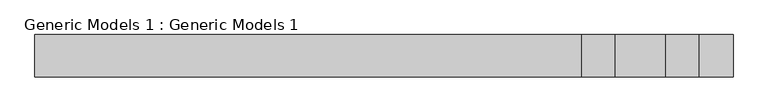
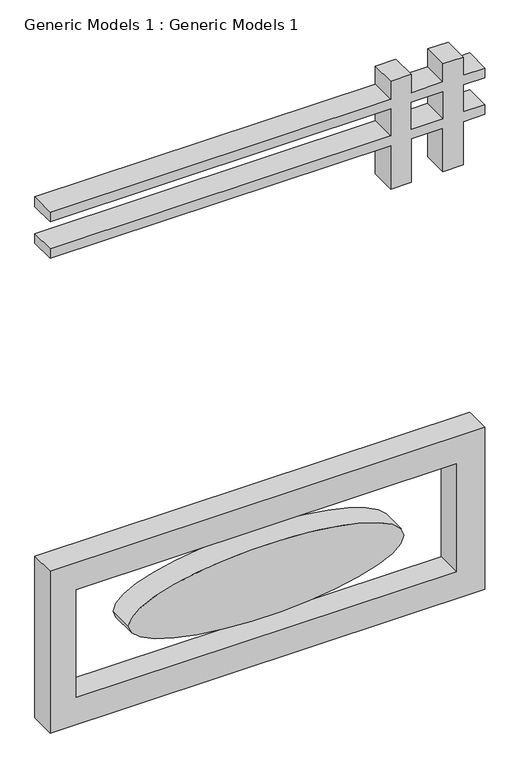
"""IFC4 building model written with IfcOpenShell, lengths in millimetres: proxy geometry, Generic Models 1 : Generic Models 1."""

from ifc_helpers import new_model, si_unit, point, frame, origin, place, context, project, spatial, polyline, ellipse_curve, trimmed, outline, extrude, source, transform, mapped, element, save
from ifc_brep_helpers import plane_surface, extruded_surface, advanced_brep


def generic_models_1_generic_models_1_d084bfd0(model_context):
    return source(origin(), model_context, "Body", "SolidModel", [
        extrude(outline(polyline([(2945.7806147, -9147.962181), (3048.0, -9147.962181), (3048.0, -9256.9307419), (2945.7806147, -9256.9307419), (2945.7806147, -9427.362181), (3048.0, -9427.362181), (3048.0, -9536.3307419), (2945.7806147, -9536.3307419), (2945.7806147, -11357.3277598), (2891.0724485, -11357.3277598), (2891.0724485, -9536.3307419), (2738.6724485, -9536.3307419), (2738.6724485, -11357.3277598), (2683.9642823, -11357.3277598), (2683.9642823, -9536.3307419), (2438.4, -9536.3307419), (2438.4, -9427.362181), (2683.9642823, -9427.362181), (2683.9642823, -9256.9307419), (2438.4, -9256.9307419), (2438.4, -9147.962181), (2683.9642823, -9147.962181), (2683.9642823, -9033.2277598), (2738.6724485, -9033.2277598), (2738.6724485, -9147.962181), (2891.0724485, -9147.962181), (2891.0724485, -9033.2277598), (2945.7806147, -9033.2277598), (2945.7806147, -9147.962181)]), holes=[polyline([(2738.6724485, -9427.362181), (2891.0724485, -9427.362181), (2891.0724485, -9256.9307419), (2738.6724485, -9256.9307419), (2738.6724485, -9427.362181)])]), frame((0.0, 2074.8342801, 0.0), z_axis=(0.0, 1.0, 0.0), x_axis=(0.0, 0.0, 1.0)), (0.0, 0.0, 1.0), 140.9087581),
        advanced_brep(
        [(-10938.2277598, 2074.8342801, 457.2), (-9465.0277598, 2074.8342801, 457.2), (-10938.2277598, 2215.7430382, 457.2), (-9465.0277598, 2215.7430382, 457.2)],
        [
            (0, 1, ellipse_curve(frame((-10201.6277598, 2074.8342801, 457.2), z_axis=(0.0, -1.0, 0.0), x_axis=(1.0, 0.0, 0.0)), 736.6, 203.2)),
            (1, 0, ellipse_curve(frame((-10201.6277598, 2074.8342801, 457.2), z_axis=(0.0, -1.0, 0.0), x_axis=(1.0, 0.0, 0.0)), 736.6, 203.2)),
            (2, 3, ellipse_curve(frame((-10201.6277598, 2215.7430382, 457.2), z_axis=(0.0, 1.0, 0.0), x_axis=(1.0, 0.0, 0.0)), 736.6, 203.2)),
            (3, 2, ellipse_curve(frame((-10201.6277598, 2215.7430382, 457.2), z_axis=(0.0, 1.0, 0.0), x_axis=(1.0, 0.0, 0.0)), 736.6, 203.2)),
            (0, 2),
            (3, 1),
        ],
        [
            plane_surface(frame((-9465.0277598, 2074.8342801, 457.2), z_axis=(0.0, -1.0, 0.0), x_axis=(0.0, 0.0, 1.0))),
            plane_surface(frame((-9465.0277598, 2215.7430382, 457.2), z_axis=(0.0, 1.0, 0.0), x_axis=(0.0, 0.0, -1.0))),
            extruded_surface(trimmed(ellipse_curve(frame((-10201.6277598, 2356.6517963, 457.2), z_axis=(0.0, -1.0, 0.0), x_axis=(1.0, 0.0, 0.0)), 736.6, 203.2), [point((-10938.2277598, 2356.6517963, 457.2))], [point((-9465.0277598, 2356.6517963, 457.2))], True, "CARTESIAN"), (0.0, -140.90875810000034, 0.0), 140.90875810000034),
            extruded_surface(trimmed(ellipse_curve(frame((-10201.6277598, 2356.6517963, 457.2), z_axis=(0.0, -1.0, 0.0), x_axis=(1.0, 0.0, 0.0)), 736.6, 203.2), [point((-9465.0277598, 2356.6517963, 457.2))], [point((-10938.2277598, 2356.6517963, 457.2))], True, "CARTESIAN"), (0.0, -140.90875810000034, 0.0), 140.90875810000034),
        ],
        [
            (0, [[1, 2]]),
            (1, [[3, 4]]),
            (2, [[-1, 5, -4, 6]]),
            (3, [[-2, -6, -3, -5]]),
        ],
    ),
        extrude(outline(polyline([(914.4, -11357.3277598), (0.0, -11357.3277598), (0.0, -9033.2277598), (914.4, -9033.2277598), (914.4, -11357.3277598)]), holes=[polyline([(762.0, -11217.6277598), (762.0, -9185.6277598), (152.4, -9185.6277598), (152.4, -11217.6277598), (762.0, -11217.6277598)])]), frame((0.0, 2074.8342801, 0.0), z_axis=(0.0, 1.0, 0.0), x_axis=(0.0, 0.0, 1.0)), (0.0, 0.0, 1.0), 140.9087581),
    ])


if __name__ == "__main__":
    model = new_model("IFC4")
    model_context = context("Model", 3, world=origin())
    ifc_project = project(units=[si_unit("LENGTHUNIT", "METRE", prefix="MILLI")], contexts=[model_context])
    site = spatial("IfcSite", under=ifc_project)
    building = spatial("IfcBuilding", under=site)
    placement = place(None, origin())
    generic_models_1_generic_models_1_shape = generic_models_1_generic_models_1_d084bfd0(model_context)
    element("IfcBuildingElementProxy", 1, Name="Generic Models 1 : Generic Models 1", ObjectType="Generic Models 1 : Generic Models 1", at=placement, inside=building, context=model_context, shape_type="MappedRepresentation", body=[
        mapped(generic_models_1_generic_models_1_shape, transform((0.0, 0.0, 0.0), x_axis=(1.0, 0.0, 0.0), y_axis=(0.0, 1.0, 0.0), z_axis=(0.0, 0.0, 1.0))),
    ])
    save(model, "model.ifc")
